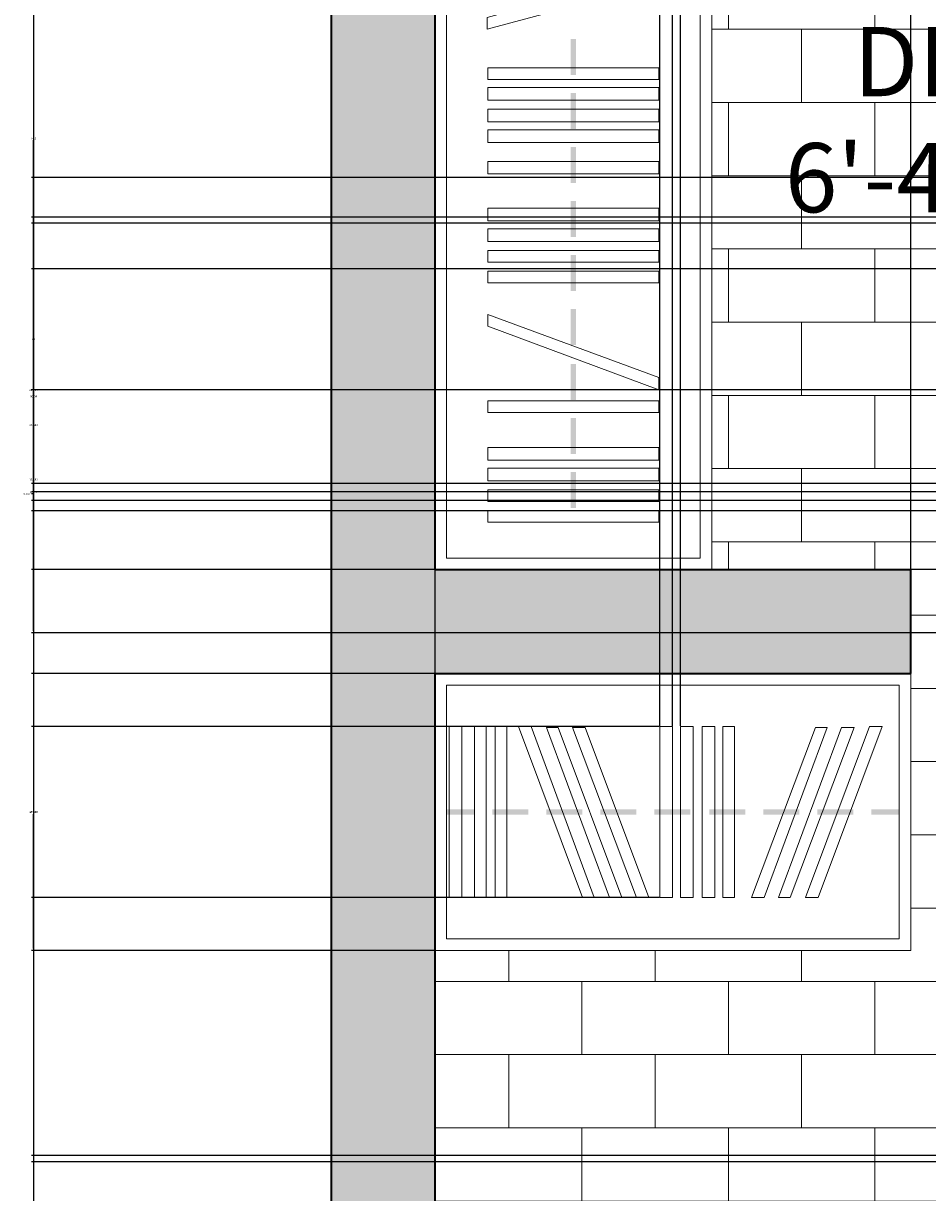
# Model space of a CAD drawing. Units: inches. Extents: x 6 to 575, y 34 to 566.
# Tile 6 of 21: x 6 to 84, y 387 to 488. Entities that reach past the tile are written whole.
import ezdxf

# ---------------------------------------------------------------- set-up
doc = ezdxf.new("R2010")
doc.units = ezdxf.units.IN
for name, color, linetype, lineweight in [('A-ANNO-DIMS', 2, 'Continuous', 18), ('A-AREA-IDEN', 6, 'Continuous', 20), ('A-FLOR-CASE', 2, 'Continuous', 18), ('A-FLOR-PATT', 252, 'Continuous', 9), ('A-WALL-PATT', 251, 'Continuous', 9), ('WALLS', 7, 'Continuous', 35)]:
    doc.layers.add(name, color=color, linetype=linetype, lineweight=lineweight)
doc.styles.add('PDF Arial Narrow', font='txt')
doc.styles.get("Standard").update_dxf_attribs({"font": 'arial.ttf'})
doc.dimstyles.get("Standard").update_dxf_attribs({"dimtxt": 0.18, "dimasz": 0.18, "dimexe": 0.18, "dimexo": 0.0625, "dimgap": 0.09, "dimtad": 0, "dimtih": 1, "dimtoh": 1, "dimdec": 4, "dimzin": 0, "dimdsep": 46, "dimtxsty": 'Standard', "dimcen": 0.09, "dimadec": 0, "dimazin": 0, "dimtfac": 1, "dimtdec": 4, "dimtofl": 0, "dimtmove": 0, "dimatfit": 3, "dimfxl": 1, "dimtolj": 1, "dimtzin": 0, "dimarcsym": 0})

# ---------------------------------------------------------------- blocks, each defined once
blk = doc.blocks.new('*D30')
at = {"layer": 'A-ANNO-DIMS', "color": 0, "lineweight": -2, "transparency": 16777216}
for p, q in [((32.6, 539.8), (6.65, 539.8)), ((6.83, 539.62), (6.83, 299.97)), ((6.83, 59.95), (6.83, 299.61)), ((197.62, 59.77), (6.65, 59.77))]:
    blk.add_line(p, q, dxfattribs=at)
at = {"layer": 'A-ANNO-DIMS', "color": 0, "transparency": 16777216}
for points in [[(6.8, 539.62), (6.86, 539.62), (6.83, 539.8)], [(6.8, 59.95), (6.86, 59.95), (6.83, 59.77)]]:
    blk.add_solid(points, dxfattribs=at)
at = {"layer": 'Defpoints', "color": 0, "transparency": 16777216}
for p in [(32.66, 539.8), (6.83, 59.77), (197.69, 59.77)]:
    blk.add_point(p, dxfattribs=at)
at = {"layer": 'A-ANNO-DIMS', "color": 0, "transparency": 16777216, "insert": (6.83, 299.79), "char_height": 0.18, "attachment_point": 5}
blk.add_mtext('\\A1;480', dxfattribs=at)
blk = doc.blocks.new('*D52')
at = {"layer": 'A-ANNO-DIMS', "color": 0, "lineweight": -2, "transparency": 16777216}
for p, q in [((437.62, 471.35), (6.65, 471.35)), ((6.83, 471.17), (6.83, 453.51)), ((6.83, 435.49), (6.83, 453.15)), ((437.62, 435.31), (6.65, 435.31))]:
    blk.add_line(p, q, dxfattribs=at)
at = {"layer": 'A-ANNO-DIMS', "color": 0, "transparency": 16777216}
for points in [[(6.8, 471.17), (6.86, 471.17), (6.83, 471.35)], [(6.8, 435.49), (6.86, 435.49), (6.83, 435.31)]]:
    blk.add_solid(points, dxfattribs=at)
at = {"layer": 'Defpoints', "color": 0, "transparency": 16777216}
for p in [(6.83, 471.35), (437.69, 471.35), (437.69, 435.31)]:
    blk.add_point(p, dxfattribs=at)
at = {"layer": 'A-ANNO-DIMS', "color": 0, "transparency": 16777216, "insert": (6.83, 453.33), "char_height": 0.18, "attachment_point": 5}
blk.add_mtext('\\A1;36.045', dxfattribs=at)
blk = doc.blocks.new('*D55')
at = {"layer": 'A-ANNO-DIMS', "color": 0, "lineweight": -2, "transparency": 16777216}
for p, q in [((41.66, 286.13), (41.66, 565.81)), ((122.56, 286.13), (122.56, 565.81)), ((41.84, 565.63), (81.79, 565.63)), ((122.38, 565.63), (82.44, 565.63))]:
    blk.add_line(p, q, dxfattribs=at)
at = {"layer": 'A-ANNO-DIMS', "color": 0, "transparency": 16777216}
for points in [[(41.84, 565.66), (41.84, 565.6), (41.66, 565.63)], [(122.38, 565.66), (122.38, 565.6), (122.56, 565.63)]]:
    blk.add_solid(points, dxfattribs=at)
at = {"layer": 'Defpoints', "color": 0, "transparency": 16777216}
for p in [(122.56, 565.63), (41.66, 286.06), (122.56, 286.06)]:
    blk.add_point(p, dxfattribs=at)
at = {"layer": 'A-ANNO-DIMS', "color": 0, "transparency": 16777216, "insert": (82.11, 565.63), "char_height": 0.18, "attachment_point": 5}
blk.add_mtext('\\A1;80.9', dxfattribs=at)
blk = doc.blocks.new('*D66')
at = {"layer": 'A-ANNO-DIMS', "color": 0, "lineweight": -2, "transparency": 16777216}
for p, q in [((41.66, 440.86), (41.66, 565.81)), ((82.89, 440.86), (82.89, 565.81)), ((41.84, 565.63), (61.88, 565.63)), ((82.71, 565.63), (62.67, 565.63))]:
    blk.add_line(p, q, dxfattribs=at)
at = {"layer": 'A-ANNO-DIMS', "color": 0, "transparency": 16777216}
for points in [[(41.84, 565.66), (41.84, 565.6), (41.66, 565.63)], [(82.71, 565.66), (82.71, 565.6), (82.89, 565.63)]]:
    blk.add_solid(points, dxfattribs=at)
at = {"layer": 'Defpoints', "color": 0, "transparency": 16777216}
for p in [(82.89, 565.63), (41.66, 440.8), (82.89, 440.8)]:
    blk.add_point(p, dxfattribs=at)
at = {"layer": 'A-ANNO-DIMS', "color": 0, "transparency": 16777216, "insert": (62.28, 565.63), "char_height": 0.18, "attachment_point": 5}
blk.add_mtext('\\A1;41.23', dxfattribs=at)
blk = doc.blocks.new('*D67')
at = {"layer": 'A-ANNO-DIMS', "color": 0, "lineweight": -2, "transparency": 16777216}
for p, q in [((82.89, 440.86), (82.89, 565.81)), ((111.66, 440.86), (111.66, 565.81)), ((83.07, 565.63), (96.81, 565.63)), ((111.48, 565.63), (97.74, 565.63))]:
    blk.add_line(p, q, dxfattribs=at)
at = {"layer": 'A-ANNO-DIMS', "color": 0, "transparency": 16777216}
for points in [[(83.07, 565.66), (83.07, 565.6), (82.89, 565.63)], [(111.48, 565.66), (111.48, 565.6), (111.66, 565.63)]]:
    blk.add_solid(points, dxfattribs=at)
at = {"layer": 'Defpoints', "color": 0, "transparency": 16777216}
for p in [(111.66, 565.63), (82.89, 440.8), (111.66, 440.8)]:
    blk.add_point(p, dxfattribs=at)
at = {"layer": 'A-ANNO-DIMS', "color": 0, "transparency": 16777216, "insert": (97.28, 565.63), "char_height": 0.18, "attachment_point": 5}
blk.add_mtext('\\A1;28.767', dxfattribs=at)
blk = doc.blocks.new('*D110')
at = {"layer": 'A-ANNO-DIMS', "color": 0, "lineweight": -2, "transparency": 16777216}
for p, q in [((41.6, 431.8), (6.65, 431.8)), ((6.83, 431.62), (6.83, 419.97)), ((6.83, 407.95), (6.83, 419.6)), ((41.56, 407.77), (6.65, 407.77))]:
    blk.add_line(p, q, dxfattribs=at)
at = {"layer": 'A-ANNO-DIMS', "color": 0, "transparency": 16777216}
for points in [[(6.8, 431.62), (6.86, 431.62), (6.83, 431.8)], [(6.8, 407.95), (6.86, 407.95), (6.83, 407.77)]]:
    blk.add_solid(points, dxfattribs=at)
at = {"layer": 'Defpoints', "color": 0, "transparency": 16777216}
for p in [(41.66, 431.8), (6.83, 407.77), (41.62, 407.77)]:
    blk.add_point(p, dxfattribs=at)
at = {"layer": 'A-ANNO-DIMS', "color": 0, "transparency": 16777216, "insert": (6.83, 419.79), "char_height": 0.18, "attachment_point": 5}
blk.add_mtext('\\A1;24.03', dxfattribs=at)
blk = doc.blocks.new('*D114')
at = {"layer": 'A-ANNO-DIMS', "color": 0, "lineweight": -2, "transparency": 16777216}
for p, q in [((61.06, 427.2), (6.65, 427.2)), ((6.83, 427.02), (6.83, 419.97)), ((6.83, 412.55), (6.83, 419.6)), ((61.06, 412.37), (6.65, 412.37))]:
    blk.add_line(p, q, dxfattribs=at)
at = {"layer": 'A-ANNO-DIMS', "color": 0, "transparency": 16777216}
for points in [[(6.8, 427.02), (6.86, 427.02), (6.83, 427.2)], [(6.8, 412.55), (6.86, 412.55), (6.83, 412.37)]]:
    blk.add_solid(points, dxfattribs=at)
at = {"layer": 'Defpoints', "color": 0, "transparency": 16777216}
for p in [(61.12, 427.2), (6.83, 412.37), (61.12, 412.37)]:
    blk.add_point(p, dxfattribs=at)
at = {"layer": 'A-ANNO-DIMS', "color": 0, "transparency": 16777216, "insert": (6.83, 419.79), "char_height": 0.18, "attachment_point": 5}
blk.add_mtext('\\A1;14.824', dxfattribs=at)
blk = doc.blocks.new('*D115')
at = {"layer": 'A-ANNO-DIMS', "color": 0, "lineweight": -2, "transparency": 16777216}
for p, q in [((61.12, 427.26), (61.12, 565.81)), ((62.22, 427.26), (62.22, 565.81)), ((60.94, 565.63), (60.76, 565.63)), ((62.4, 565.63), (62.58, 565.63))]:
    blk.add_line(p, q, dxfattribs=at)
at = {"layer": 'A-ANNO-DIMS', "color": 0, "transparency": 16777216}
for points in [[(60.94, 565.66), (60.94, 565.6), (61.12, 565.63)], [(62.4, 565.66), (62.4, 565.6), (62.22, 565.63)]]:
    blk.add_solid(points, dxfattribs=at)
at = {"layer": 'Defpoints', "color": 0, "transparency": 16777216}
for p in [(62.22, 565.63), (61.12, 427.2), (62.22, 427.2)]:
    blk.add_point(p, dxfattribs=at)
at = {"layer": 'A-ANNO-DIMS', "color": 0, "transparency": 16777216, "insert": (61.67, 565.63), "char_height": 0.18, "attachment_point": 5}
blk.add_mtext('\\A1;1.09', dxfattribs=at)
blk = doc.blocks.new('*D116')
at = {"layer": 'A-ANNO-DIMS', "color": 0, "lineweight": -2, "transparency": 16777216}
for p, q in [((61.12, 427.26), (61.12, 565.81)), ((62.92, 427.26), (62.92, 565.81)), ((61.3, 565.63), (61.71, 565.63)), ((62.74, 565.63), (62.34, 565.63))]:
    blk.add_line(p, q, dxfattribs=at)
at = {"layer": 'A-ANNO-DIMS', "color": 0, "transparency": 16777216}
for points in [[(61.3, 565.66), (61.3, 565.6), (61.12, 565.63)], [(62.74, 565.66), (62.74, 565.6), (62.92, 565.63)]]:
    blk.add_solid(points, dxfattribs=at)
at = {"layer": 'Defpoints', "color": 0, "transparency": 16777216}
for p in [(62.92, 565.63), (61.12, 427.2), (62.92, 427.2)]:
    blk.add_point(p, dxfattribs=at)
at = {"layer": 'A-ANNO-DIMS', "color": 0, "transparency": 16777216, "insert": (62.02, 565.63), "char_height": 0.18, "attachment_point": 5}
blk.add_mtext('\\A1;1.79', dxfattribs=at)
blk = doc.blocks.new('*D117')
at = {"layer": 'A-ANNO-DIMS', "color": 0, "lineweight": -2, "transparency": 16777216}
for p, q in [((41.6, 515.59), (6.65, 515.59)), ((6.83, 515.41), (6.83, 478.38)), ((6.83, 440.98), (6.83, 478.02)), ((41.6, 440.8), (6.65, 440.8))]:
    blk.add_line(p, q, dxfattribs=at)
at = {"layer": 'A-ANNO-DIMS', "color": 0, "transparency": 16777216}
for points in [[(6.8, 515.41), (6.86, 515.41), (6.83, 515.59)], [(6.8, 440.98), (6.86, 440.98), (6.83, 440.8)]]:
    blk.add_solid(points, dxfattribs=at)
at = {"layer": 'Defpoints', "color": 0, "transparency": 16777216}
for p in [(6.83, 515.59), (41.66, 515.59), (41.66, 440.8)]:
    blk.add_point(p, dxfattribs=at)
at = {"layer": 'A-ANNO-DIMS', "color": 0, "transparency": 16777216, "insert": (6.83, 478.2), "char_height": 0.18, "attachment_point": 5}
blk.add_mtext('\\A1;74.8', dxfattribs=at)
blk = doc.blocks.new('*D132')
at = {"layer": 'A-ANNO-DIMS', "color": 0, "lineweight": -2, "transparency": 16777216}
for p, q in [((288.54, 390), (6.65, 390)), ((6.83, 389.82), (6.83, 366.19)), ((6.83, 342.19), (6.83, 365.82)), ((288.54, 342.01), (6.65, 342.01))]:
    blk.add_line(p, q, dxfattribs=at)
at = {"layer": 'A-ANNO-DIMS', "color": 0, "transparency": 16777216}
for points in [[(6.8, 389.82), (6.86, 389.82), (6.83, 390)], [(6.8, 342.19), (6.86, 342.19), (6.83, 342.01)]]:
    blk.add_solid(points, dxfattribs=at)
at = {"layer": 'Defpoints', "color": 0, "transparency": 16777216}
for p in [(6.83, 390), (288.6, 390), (288.6, 342.01)]:
    blk.add_point(p, dxfattribs=at)
at = {"layer": 'A-ANNO-DIMS', "color": 0, "transparency": 16777216, "insert": (6.83, 366), "char_height": 0.18, "attachment_point": 5}
blk.add_mtext('\\A1;47.98', dxfattribs=at)
blk = doc.blocks.new('*D136')
at = {"layer": 'A-ANNO-DIMS', "color": 0, "lineweight": -2, "transparency": 16777216}
for p, q in [((206.62, 389.45), (6.65, 389.45)), ((6.83, 389.27), (6.83, 350.19)), ((6.83, 310.75), (6.83, 349.83)), ((206.62, 310.57), (6.65, 310.57))]:
    blk.add_line(p, q, dxfattribs=at)
at = {"layer": 'A-ANNO-DIMS', "color": 0, "transparency": 16777216}
for points in [[(6.8, 389.27), (6.86, 389.27), (6.83, 389.45)], [(6.8, 310.75), (6.86, 310.75), (6.83, 310.57)]]:
    blk.add_solid(points, dxfattribs=at)
at = {"layer": 'Defpoints', "color": 0, "transparency": 16777216}
for p in [(6.83, 389.45), (206.68, 389.45), (206.68, 310.57)]:
    blk.add_point(p, dxfattribs=at)
at = {"layer": 'A-ANNO-DIMS', "color": 0, "transparency": 16777216, "insert": (6.83, 350.01), "char_height": 0.18, "attachment_point": 5}
blk.add_mtext('\\A1;78.88', dxfattribs=at)
blk = doc.blocks.new('*D186')
at = {"layer": 'A-ANNO-DIMS', "color": 0, "lineweight": -2, "transparency": 16777216}
for p, q in [((197.6, 470.84), (6.65, 470.84)), ((6.83, 470.66), (6.83, 456)), ((6.83, 440.98), (6.83, 455.64)), ((176.61, 440.8), (6.65, 440.8))]:
    blk.add_line(p, q, dxfattribs=at)
at = {"layer": 'A-ANNO-DIMS', "color": 0, "transparency": 16777216}
for points in [[(6.8, 470.66), (6.86, 470.66), (6.83, 470.84)], [(6.8, 440.98), (6.86, 440.98), (6.83, 440.8)]]:
    blk.add_solid(points, dxfattribs=at)
at = {"layer": 'Defpoints', "color": 0, "transparency": 16777216}
for p in [(6.83, 470.84), (197.66, 470.84), (176.67, 440.8)]:
    blk.add_point(p, dxfattribs=at)
at = {"layer": 'A-ANNO-DIMS', "color": 0, "transparency": 16777216, "insert": (6.83, 455.82), "char_height": 0.18, "attachment_point": 5}
blk.add_mtext('\\A1;30.04', dxfattribs=at)
blk = doc.blocks.new('*D188')
at = {"layer": 'A-ANNO-DIMS', "color": 0, "lineweight": -2, "transparency": 16777216}
for p, q in [((187.14, 466.88), (6.65, 466.88)), ((6.83, 466.7), (6.83, 456.56)), ((6.83, 446.07), (6.83, 456.2)), ((187.02, 445.89), (6.65, 445.89))]:
    blk.add_line(p, q, dxfattribs=at)
at = {"layer": 'A-ANNO-DIMS', "color": 0, "transparency": 16777216}
for points in [[(6.8, 466.7), (6.86, 466.7), (6.83, 466.88)], [(6.8, 446.07), (6.86, 446.07), (6.83, 445.89)]]:
    blk.add_solid(points, dxfattribs=at)
at = {"layer": 'Defpoints', "color": 0, "transparency": 16777216}
for p in [(6.83, 466.88), (187.2, 466.88), (187.08, 445.89)]:
    blk.add_point(p, dxfattribs=at)
at = {"layer": 'A-ANNO-DIMS', "color": 0, "transparency": 16777216, "insert": (6.83, 456.38), "char_height": 0.18, "attachment_point": 5}
blk.add_mtext('\\A1;20.987', dxfattribs=at)
blk = doc.blocks.new('*D189')
at = {"layer": 'A-ANNO-DIMS', "color": 0, "lineweight": -2, "transparency": 16777216}
for p, q in [((187.08, 456.38), (6.65, 456.38)), ((6.83, 456.2), (6.83, 448.77)), ((6.83, 440.98), (6.83, 448.41)), ((197.6, 440.8), (6.65, 440.8))]:
    blk.add_line(p, q, dxfattribs=at)
at = {"layer": 'A-ANNO-DIMS', "color": 0, "transparency": 16777216}
for points in [[(6.8, 456.2), (6.86, 456.2), (6.83, 456.38)], [(6.8, 440.98), (6.86, 440.98), (6.83, 440.8)]]:
    blk.add_solid(points, dxfattribs=at)
at = {"layer": 'Defpoints', "color": 0, "transparency": 16777216}
for p in [(6.83, 456.38), (187.14, 456.38), (197.66, 440.8)]:
    blk.add_point(p, dxfattribs=at)
at = {"layer": 'A-ANNO-DIMS', "color": 0, "transparency": 16777216, "insert": (6.83, 448.59), "char_height": 0.18, "attachment_point": 5}
blk.add_mtext('\\A1;15.582', dxfattribs=at)
blk = doc.blocks.new('*D197')
at = {"layer": 'A-ANNO-DIMS', "color": 0, "lineweight": -2, "transparency": 16777216}
for p, q in [((117.6, 446.8), (6.65, 446.8)), ((6.83, 446.62), (6.83, 443.98)), ((6.83, 440.98), (6.83, 443.62)), ((117.6, 440.8), (6.65, 440.8))]:
    blk.add_line(p, q, dxfattribs=at)
at = {"layer": 'A-ANNO-DIMS', "color": 0, "transparency": 16777216}
for points in [[(6.8, 446.62), (6.86, 446.62), (6.83, 446.8)], [(6.8, 440.98), (6.86, 440.98), (6.83, 440.8)]]:
    blk.add_solid(points, dxfattribs=at)
at = {"layer": 'Defpoints', "color": 0, "transparency": 16777216}
for p in [(6.83, 446.8), (117.66, 446.8), (117.66, 440.8)]:
    blk.add_point(p, dxfattribs=at)
at = {"layer": 'A-ANNO-DIMS', "color": 0, "transparency": 16777216, "insert": (6.83, 443.8), "char_height": 0.18, "attachment_point": 5}
blk.add_mtext('\\A1;6', dxfattribs=at)
blk = doc.blocks.new('*D198')
at = {"layer": 'A-ANNO-DIMS', "color": 0, "lineweight": -2, "transparency": 16777216}
for p, q in [((117.6, 474.8), (6.65, 474.8)), ((6.83, 474.62), (6.83, 460.98)), ((6.83, 446.98), (6.83, 460.62)), ((117.6, 446.8), (6.65, 446.8))]:
    blk.add_line(p, q, dxfattribs=at)
at = {"layer": 'A-ANNO-DIMS', "color": 0, "transparency": 16777216}
for points in [[(6.8, 474.62), (6.86, 474.62), (6.83, 474.8)], [(6.8, 446.98), (6.86, 446.98), (6.83, 446.8)]]:
    blk.add_solid(points, dxfattribs=at)
at = {"layer": 'Defpoints', "color": 0, "transparency": 16777216}
for p in [(6.83, 474.8), (117.66, 474.8), (117.66, 446.8)]:
    blk.add_point(p, dxfattribs=at)
at = {"layer": 'A-ANNO-DIMS', "color": 0, "transparency": 16777216, "insert": (6.83, 460.8), "char_height": 0.18, "attachment_point": 5}
blk.add_mtext('\\A1;28', dxfattribs=at)
blk = doc.blocks.new('*D203')
at = {"layer": 'A-ANNO-DIMS', "color": 0, "lineweight": -2, "transparency": 16777216}
for p, q in [((117.6, 448.28), (6.65, 448.28)), ((6.83, 448.1), (6.83, 447.72)), ((6.83, 446.98), (6.83, 447.36)), ((117.6, 446.8), (6.65, 446.8))]:
    blk.add_line(p, q, dxfattribs=at)
at = {"layer": 'A-ANNO-DIMS', "color": 0, "transparency": 16777216}
for points in [[(6.8, 448.1), (6.86, 448.1), (6.83, 448.28)], [(6.8, 446.98), (6.86, 446.98), (6.83, 446.8)]]:
    blk.add_solid(points, dxfattribs=at)
at = {"layer": 'Defpoints', "color": 0, "transparency": 16777216}
for p in [(6.83, 448.28), (117.66, 448.28), (117.66, 446.8)]:
    blk.add_point(p, dxfattribs=at)
at = {"layer": 'A-ANNO-DIMS', "color": 0, "transparency": 16777216, "insert": (6.83, 447.54), "char_height": 0.18, "attachment_point": 5}
blk.add_mtext('\\A1;1.474', dxfattribs=at)
blk = doc.blocks.new('*D204')
at = {"layer": 'A-ANNO-DIMS', "color": 0, "lineweight": -2, "transparency": 16777216}
for p, q in [((119.07, 448.28), (6.65, 448.28)), ((6.83, 448.1), (6.83, 447.72)), ((119.07, 447.54), (6.65, 447.54)), ((6.83, 447.36), (6.65, 447.36)), ((6.83, 447.54), (6.83, 447.36))]:
    blk.add_line(p, q, dxfattribs=at)
at = {"layer": 'A-ANNO-DIMS', "color": 0, "transparency": 16777216}
for points in [[(6.8, 448.1), (6.86, 448.1), (6.83, 448.28)], [(6.8, 447.72), (6.86, 447.72), (6.83, 447.54)]]:
    blk.add_solid(points, dxfattribs=at)
at = {"layer": 'Defpoints', "color": 0, "transparency": 16777216}
for p in [(119.13, 448.28), (6.83, 447.54), (119.13, 447.54)]:
    blk.add_point(p, dxfattribs=at)
at = {"layer": 'A-ANNO-DIMS', "color": 0, "transparency": 16777216, "insert": (6.25, 447.36), "char_height": 0.18, "attachment_point": 5}
blk.add_mtext('\\A1;0.737', dxfattribs=at)

msp = doc.modelspace()

# ---------------------------------------------------------------- hatches: boundary and pattern name
at = {"layer": 'A-FLOR-PATT'}
h = msp.add_hatch(dxfattribs=at)
h.set_pattern_fill('BRICK', color=256)
h.set_pattern_definition([(0, (-98.035, 170.1465), (0, 6.35), []), (90, (-98.035, 170.147), (-12.7, 8e-16), [6.35, -6.35]), (90, (-91.685, 170.147), (-12.7, 8e-16), [-6.35, 6.35])])
h.paths.add_polyline_path([(180.8711, 269.7588), (182.4439, 270.6668), (182.4628, 270.6341, -0.11619827), (201.8275, 275.5902), (201.8275, 276.801), (197.6586, 276.801), (197.6586, 293.1641), (182.6401, 293.1641), (182.6401, 348.324), (197.6586, 348.324), (197.6586, 407.7709), (112.8513, 407.7709), (112.8513, 431.801), (111.6586, 431.801), (111.6586, 440.801), (117.6586, 440.801), (117.6586, 446.801), (117.6586, 448.2751), (117.6586, 473.3269), (117.6586, 474.801), (117.6586, 515.5941), (100.2533, 515.5941, -1), (83.0548, 515.5941), (65.6494, 515.5941), (65.6494, 440.801), (82.8918, 440.801), (82.8918, 431.801), (82.8918, 407.7709), (41.6586, 407.7709), (41.6586, 379.0637), (62.6459, 379.0637), (62.6459, 358.0764), (122.565, 358.0764), (122.565, 286.0643), (62.6459, 286.0643), (62.6459, 265.077), (41.6586, 265.077), (41.6586, 224.801), (41.6586, 212.801), (71.6586, 212.801), (167.6586, 212.801), (197.6586, 212.801), (197.6586, 230.801), (201.8157, 230.801), (201.8157, 233.4817)])
h.paths.add_polyline_path([(133.3414, 245.1275), (133.3317, 245.1352), (133.3317, 245.104)], flags=16)
h.paths.add_polyline_path([(133.3317, 222.1662), (85.3496, 222.1662), (85.3496, 243.7443, -0.50090726), (87.1831, 246.1963), (107.4292, 246.1963), (111.2522, 246.1963), (131.4202, 246.1963, -0.41421356), (133.3317, 244.2848)], flags=16)
h.paths.add_polyline_path([(72.7105, 244.4018), (72.7105, 220.3718), (48.6804, 220.3718), (48.6804, 244.4018)], flags=16)
h.paths.add_polyline_path([(71.7466, 237.8955, -1), (59.8096, 237.8955, -1)], flags=0)
at = {"layer": 'A-WALL-PATT'}
h = msp.add_hatch(color=256, dxfattribs=at)
h.dxf.hatch_style = 1
h.paths.add_polyline_path([(160.6586, 539.801), (32.6586, 539.801), (32.6586, 272.801), (41.6586, 272.801), (41.6586, 286.0643), (41.6586, 358.0764), (41.6586, 379.0637), (41.6586, 407.7709), (41.6194, 407.7709), (41.6194, 431.801), (82.8918, 431.801), (82.8918, 440.801), (65.6494, 440.801), (65.6494, 440.7732), (41.6194, 440.7732), (41.6194, 515.5941), (41.6586, 530.801), (117.6586, 530.801), (117.6586, 474.801), (120.6068, 474.801), (121.6586, 474.801), (121.6586, 530.801), (137.4275, 530.801), (137.4275, 530.8356), (141.2505, 530.8356), (160.6586, 530.801)])
h.paths.add_polyline_path([(71.6586, 212.801), (41.6586, 212.801), (41.6586, 224.801), (32.6586, 224.801), (32.6586, 203.801), (71.6586, 203.801)])
h.paths.add_polyline_path([(206.6586, 215.801), (246.6586, 215.801), (246.6586, 224.801), (206.6586, 224.801), (206.6586, 230.801), (201.8157, 230.801), (197.6586, 230.801), (197.6586, 212.801), (167.6586, 212.801), (167.6586, 203.801), (206.6586, 203.801)])
h.paths.add_polyline_path([(383.6586, 224.801), (334.6586, 224.801), (334.6586, 215.801), (374.6586, 215.801), (374.6586, 203.801), (384.0753, 203.801), (407.6586, 203.801), (407.6586, 212.801), (383.6586, 212.801)])
h.paths.add_polyline_path([(548.6586, 270.801), (539.6586, 270.801), (539.6586, 212.801), (515.6586, 212.801), (515.6586, 203.801), (548.6586, 203.801)])
h.paths.add_polyline_path([(548.6586, 412.801), (545.7108, 412.801), (539.6586, 412.801), (539.6586, 382.801), (433.708, 382.801), (433.708, 378.801), (539.6586, 378.801), (539.6586, 366.801), (548.6586, 366.801)])
h.paths.add_polyline_path([(548.6586, 539.801), (455.9436, 539.801), (455.9436, 530.801), (539.6586, 530.801), (539.6586, 440.801), (548.6586, 440.801)])
h.paths.add_polyline_path([(407.9436, 539.801), (362.6586, 539.801), (362.6586, 530.801), (374.6586, 530.801), (374.6586, 452.801), (354.6586, 452.801), (354.6586, 448.801), (374.6586, 448.801), (374.6586, 278.801), (383.6586, 278.801), (383.6586, 530.801), (407.9436, 530.801)])
h.paths.add_polyline_path([(338.6586, 539.801), (320.6586, 539.801), (320.6586, 530.801), (322.6586, 530.801), (322.6586, 448.801), (326.6586, 448.801), (326.6586, 530.801), (338.6586, 530.801)])
h.paths.add_polyline_path([(272.6586, 539.801), (184.6586, 539.801), (184.6586, 530.801), (197.6586, 530.801), (197.6586, 440.801), (176.6714, 440.801), (121.6586, 440.801), (121.6586, 446.801), (117.6586, 446.801), (117.6586, 440.801), (111.6586, 440.801), (111.6586, 431.801), (197.6586, 431.801), (197.6586, 407.7709), (197.6586, 276.801), (206.6586, 276.801), (206.6586, 530.801), (272.6586, 530.801)])

# ---------------------------------------------------------------- linework, layer by layer
at = {"layer": 'A-FLOR-CASE'}
for points in [[(41.6194, 515.5941), (41.6194, 440.7732), (65.6494, 440.7732), (65.6494, 515.5941)], [(42.6336, 514.6578), (42.6336, 441.7875), (64.6352, 441.7875), (64.6352, 514.6578)], [(46.1445, 487.663), (60.9683, 491.642), (60.9683, 492.7343), (46.1445, 488.6773)], [(46.2226, 484.3082), (61.0463, 484.3082), (61.0463, 483.2939), (46.2226, 483.2939)], [(46.2226, 482.5918), (61.0463, 482.5918), (61.0463, 481.4995), (46.2226, 481.4995)], [(46.2226, 480.7193), (61.0463, 480.7193), (61.0463, 479.627), (46.2226, 479.627)], [(46.2226, 478.9248), (61.0463, 478.9248), (61.0463, 477.8326), (46.2226, 477.8326)], [(46.2226, 476.1942), (61.0463, 476.1942), (61.0463, 475.1019), (46.2226, 475.1019)], [(46.2226, 472.1371), (61.0463, 472.1371), (61.0463, 471.0449), (46.2226, 471.0449)], [(46.2226, 470.3427), (61.0463, 470.3427), (61.0463, 469.2504), (46.2226, 469.2504)], [(46.2226, 468.4702), (61.0463, 468.4702), (61.0463, 467.456), (46.2226, 467.456)], [(46.2226, 466.6758), (61.0463, 466.6758), (61.0463, 465.6615), (46.2226, 465.6615)], [(46.2226, 462.9308), (61.0463, 457.4694), (61.0463, 456.3772), (46.2226, 461.9166)], [(46.2226, 455.4409), (61.0463, 455.4409), (61.0463, 454.4267), (46.2226, 454.4267)], [(46.2226, 451.3839), (61.0463, 451.3839), (61.0463, 450.2916), (46.2226, 450.2916)], [(46.2226, 449.5895), (61.0463, 449.5895), (61.0463, 448.4972), (46.2226, 448.4972)], [(46.2226, 447.717), (61.0463, 447.717), (61.0463, 446.7027), (46.2226, 446.7027)], [(46.2226, 445.9225), (61.0463, 445.9225), (61.0463, 444.9083), (46.2226, 444.9083)], [(41.6194, 407.7709), (82.8918, 407.7709), (82.8918, 431.801), (41.6194, 431.801)], [(42.6336, 408.7852), (81.8775, 408.7852), (81.8775, 430.7867), (42.6336, 430.7867)], [(42.8677, 412.3741), (42.8677, 427.1978), (43.96, 427.1978), (43.96, 412.3741)], [(45.0523, 412.3741), (45.0523, 427.1978), (46.0665, 427.1978), (46.0665, 412.3741)], [(46.8467, 412.3741), (46.8467, 427.1978), (47.861, 427.1978), (47.861, 412.3741)], [(55.4289, 412.3741), (49.9675, 427.1978), (48.8752, 427.1978), (54.4146, 412.3741)], [(57.8475, 412.3741), (52.3081, 427.1198), (51.2938, 427.1198), (56.7552, 412.3741)], [(60.1881, 412.3741), (54.6487, 427.1198), (53.5564, 427.1198), (59.0958, 412.3741)], [(61.1243, 412.3741), (61.1243, 427.1978), (62.2166, 427.1978), (62.2166, 412.3741)], [(62.9188, 412.3741), (62.9188, 427.1978), (64.011, 427.1978), (64.011, 412.3741)], [(64.7912, 412.3741), (64.7912, 427.1978), (65.8835, 427.1978), (65.8835, 412.3741)], [(66.5857, 412.3741), (66.5857, 427.1978), (67.5999, 427.1978), (67.5999, 412.3741)], [(69.0823, 412.3741), (74.6217, 427.1198), (75.636, 427.1198), (70.1746, 412.3741)], [(71.4229, 412.3741), (76.8843, 427.1198), (77.9765, 427.1198), (72.4371, 412.3741)], [(73.7635, 412.3741), (79.3029, 427.1978), (80.3951, 427.1978), (74.8558, 412.3741)]]:
    msp.add_lwpolyline(points, close=True, dxfattribs=at)
msp.add_lwpolyline([(42.6336, 420.02), (42.6336, 419.5519)], dxfattribs=at)
at = {"layer": 'A-FLOR-CASE', "transparency": 33554559}
for points in [[(53.4004, 483.684), (53.8685, 483.684), (53.4004, 486.8048)], [(53.8685, 483.684), (53.4004, 486.8048), (53.8685, 486.8048)], [(53.4004, 479.0029), (53.8685, 479.0029), (53.4004, 482.1236)], [(53.8685, 479.0029), (53.4004, 482.1236), (53.8685, 482.1236)], [(53.4004, 474.3217), (53.8685, 474.3217), (53.4004, 477.4425)], [(53.8685, 474.3217), (53.4004, 477.4425), (53.8685, 477.4425)], [(53.4004, 469.6405), (53.8685, 469.6405), (53.4004, 472.7613)], [(53.8685, 469.6405), (53.4004, 472.7613), (53.8685, 472.7613)], [(53.4004, 464.9593), (53.8685, 464.9593), (53.4004, 468.0801)], [(53.8685, 464.9593), (53.4004, 468.0801), (53.8685, 468.0801)], [(53.4004, 460.2781), (53.8685, 460.2781), (53.4004, 463.3989)], [(53.8685, 460.2781), (53.4004, 463.3989), (53.8685, 463.3989)], [(53.4004, 455.519), (53.8685, 455.519), (53.4004, 458.6397)], [(53.8685, 455.519), (53.4004, 458.6397), (53.8685, 458.6397)], [(53.4004, 450.8378), (53.8685, 450.8378), (53.4004, 453.9586)], [(53.8685, 450.8378), (53.4004, 453.9586), (53.8685, 453.9586)], [(53.4004, 446.1566), (53.8685, 446.1566), (53.4004, 449.2774)], [(53.8685, 446.1566), (53.4004, 449.2774), (53.8685, 449.2774)], [(45.0523, 419.5519), (45.0523, 420.02), (42.6336, 419.5519)], [(45.0523, 420.02), (42.6336, 419.5519), (42.6336, 420.02)], [(49.7334, 419.5519), (49.7334, 420.02), (46.6127, 419.5519)], [(49.7334, 420.02), (46.6127, 419.5519), (46.6127, 420.02)], [(54.4146, 419.5519), (54.4146, 420.02), (51.2938, 419.5519)], [(54.4146, 420.02), (51.2938, 419.5519), (51.2938, 420.02)], [(59.0958, 419.5519), (59.0958, 420.02), (55.975, 419.5519)], [(59.0958, 420.02), (55.975, 419.5519), (55.975, 420.02)], [(63.777, 419.5519), (63.777, 420.02), (60.6562, 419.5519)], [(63.777, 420.02), (60.6562, 419.5519), (60.6562, 420.02)], [(68.5362, 419.5519), (68.5362, 420.02), (65.4154, 419.5519)], [(68.5362, 420.02), (65.4154, 419.5519), (65.4154, 420.02)], [(73.2173, 419.5519), (73.2173, 420.02), (70.0966, 419.5519)], [(73.2173, 420.02), (70.0966, 419.5519), (70.0966, 420.02)], [(77.8985, 419.5519), (77.8985, 420.02), (74.7777, 419.5519)], [(77.8985, 420.02), (74.7777, 419.5519), (74.7777, 420.02)], [(81.8775, 419.5519), (81.8775, 420.02), (79.4589, 419.5519)], [(81.8775, 420.02), (79.4589, 419.5519), (79.4589, 420.02)]]:
    msp.add_solid(points, dxfattribs=at)
at = {"layer": 'WALLS'}
for p, q in [((32.6586, 272.801), (32.6586, 539.801)), ((41.6586, 440.801), (41.6586, 530.801)), ((41.6586, 440.801), (82.8918, 440.801)), ((82.8918, 431.801), (82.8918, 440.801)), ((41.6586, 431.801), (82.8918, 431.801)), ((41.6586, 272.801), (41.6586, 431.801))]:
    msp.add_line(p, q, dxfattribs=at)

# ---------------------------------------------------------------- texts
at = {"layer": 'A-AREA-IDEN', "attachment_point": 4, "style": 'PDF Arial Narrow'}
for s, insert, char_height in [('DRESS', (77.9064, 484.0646), 6.0005), ('6\'-4" X 7\'-6"', (71.9766, 473.9997), 6.000503)]:
    msp.add_mtext(s, dxfattribs=dict(at, insert=insert, char_height=char_height))

# ---------------------------------------------------------------- dimensions: what is measured, and where the dimension line sits
at = {"layer": 'A-ANNO-DIMS'}
for base, p1, p2, override, picture, middle in [((122.565, 565.631), (41.6586, 286.0643), (122.565, 286.0643), {"dimdec": 1, "dimlfac": 1, "dimrnd": 0, "dimzin": 0, "dimdsep": 46, "dimlunit": 2}, '*D55', (82.1118, 565.631)), ((82.8918, 565.631), (41.6586, 440.801), (82.8918, 440.801), {"dimdec": 2, "dimlfac": 1, "dimrnd": 0, "dimzin": 0, "dimdsep": 46, "dimlunit": 2}, '*D66', (62.2752, 565.631)), ((62.2166, 565.631), (61.1243, 427.1978), (62.2166, 427.1978), {"dimdec": 2, "dimlfac": 1, "dimrnd": 0, "dimzin": 0, "dimdsep": 46, "dimlunit": 2}, '*D115', (61.6704, 565.631)), ((62.9188, 565.631), (61.1243, 427.1978), (62.9188, 427.1978), {"dimdec": 2, "dimlfac": 1, "dimrnd": 0, "dimzin": 0, "dimdsep": 46, "dimlunit": 2}, '*D116', (62.0215, 565.631)), ((111.6586, 565.631), (82.8918, 440.801), (111.6586, 440.801), {"dimdec": 3, "dimlfac": 1, "dimrnd": 0, "dimzin": 0, "dimdsep": 46, "dimlunit": 2}, '*D67', (97.2752, 565.631))]:
    dim = msp.add_linear_dim(base=base, p1=p1, p2=p2, dimstyle='Standard', override=override, dxfattribs=at)
    dim.commit()
    dim.dimension.update_dxf_attribs({"geometry": picture, "text_midpoint": middle})
for base, p1, p2, override, picture, middle in [((6.8286, 59.7747), (32.6586, 539.801), (197.6872, 59.7747), {"dimdec": 0, "dimlfac": 1, "dimrnd": 0, "dimzin": 0, "dimdsep": 46, "dimlunit": 2}, '*D30', (6.8286, 299.7878)), ((6.8286, 515.5941), (41.6586, 440.801), (41.6586, 515.5941), {"dimdec": 1, "dimlfac": 1, "dimrnd": 0, "dimzin": 0, "dimdsep": 46, "dimlunit": 2}, '*D117', (6.8286, 478.1975)), ((6.8286, 474.801), (117.6586, 446.801), (117.6586, 474.801), {"dimdec": 0, "dimlfac": 1, "dimrnd": 0, "dimzin": 0, "dimdsep": 46, "dimlunit": 2}, '*D198', (6.8286, 460.801)), ((6.8286, 471.3533), (437.687, 435.3082), (437.687, 471.3533), {"dimdec": 3, "dimlfac": 1, "dimrnd": 0, "dimzin": 0, "dimdsep": 46, "dimlunit": 2}, '*D52', (6.8286, 453.3307)), ((6.8286, 470.8385), (176.6714, 440.801), (197.6586, 470.8385), {"dimdec": 2, "dimlfac": 1, "dimrnd": 0, "dimzin": 0, "dimdsep": 46, "dimlunit": 2}, '*D186', (6.8286, 455.8198)), ((6.8286, 466.8767), (187.0809, 445.8894), (187.2036, 466.8767), {"dimdec": 3, "dimlfac": 1, "dimrnd": 0, "dimzin": 0, "dimdsep": 46, "dimlunit": 2}, '*D188', (6.8286, 456.3831)), ((6.8286, 456.3831), (197.6586, 440.801), (187.1423, 456.3831), {"dimdec": 3, "dimlfac": 1, "dimrnd": 0, "dimzin": 0, "dimdsep": 46, "dimlunit": 2}, '*D189', (6.8286, 448.592)), ((6.8286, 447.538), (119.1327, 448.2751), (119.1327, 447.538), {"dimdec": 3, "dimlfac": 1, "dimrnd": 0, "dimzin": 0, "dimdsep": 46, "dimlunit": 2}, '*D204', (6.2549, 447.358)), ((6.8286, 448.2751), (117.6586, 446.801), (117.6586, 448.2751), {"dimdec": 3, "dimlfac": 1, "dimrnd": 0, "dimzin": 0, "dimdsep": 46, "dimlunit": 2}, '*D203', (6.8286, 447.538)), ((6.8286, 446.801), (117.6586, 440.801), (117.6586, 446.801), {"dimdec": 0, "dimlfac": 1, "dimrnd": 0, "dimzin": 0, "dimdsep": 46, "dimlunit": 2}, '*D197', (6.8286, 443.801)), ((6.8286, 407.7709), (41.6586, 431.801), (41.6194, 407.7709), {"dimdec": 2, "dimlfac": 1, "dimrnd": 0, "dimzin": 0, "dimdsep": 46, "dimlunit": 2}, '*D110', (6.8286, 419.786)), ((6.8286, 412.3741), (61.1243, 427.1978), (61.1243, 412.3741), {"dimdec": 3, "dimlfac": 1, "dimrnd": 0, "dimzin": 0, "dimdsep": 46, "dimlunit": 2}, '*D114', (6.8286, 419.786)), ((6.8286, 389.9952), (288.603, 342.0131), (288.603, 389.9952), {"dimdec": 2, "dimlfac": 1, "dimrnd": 0, "dimzin": 0, "dimdsep": 46, "dimlunit": 2}, '*D132', (6.8286, 366.0042)), ((6.8286, 389.449), (206.6824, 310.5712), (206.6824, 389.449), {"dimdec": 2, "dimlfac": 1, "dimrnd": 0, "dimzin": 0, "dimdsep": 46, "dimlunit": 2}, '*D136', (6.8286, 350.0101))]:
    dim = msp.add_linear_dim(base=base, p1=p1, p2=p2, angle=90, dimstyle='Standard', override=override, dxfattribs=at)
    dim.commit()
    dim.dimension.update_dxf_attribs({"geometry": picture, "text_midpoint": middle})

doc.saveas('drawing.dxf')
